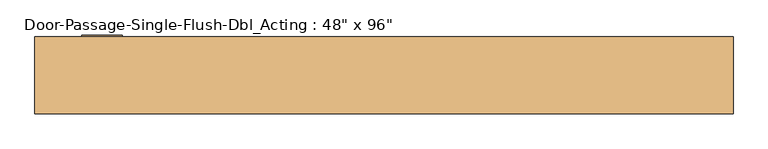
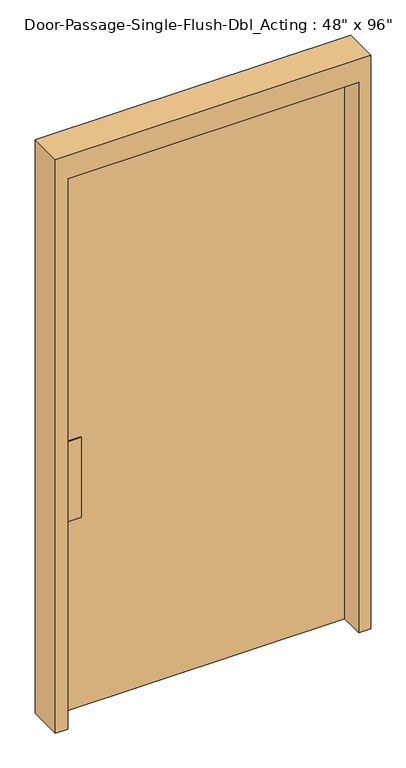
"""IFC4 building model written with IfcOpenShell, lengths in millimetres: door geometry."""

from ifc_helpers import new_model, si_unit, frame, origin, origin_with_axes, place, context, project, spatial, polyline, outline, extrude, source, transform, mapped, element, save


def door_bb6275b8(model_context):
    return source(origin(), model_context, "Body", "SweptSolid", [
        extrude(outline(polyline([(-571.5, 85.725), (-571.5, 88.9), (-495.3, 88.9), (-495.3, 85.725), (-571.5, 85.725)])), frame((0.0, 0.0, 838.2), z_axis=(0.0, 0.0, 1.0), x_axis=(1.0, 0.0, 0.0)), (0.0, 0.0, 1.0), 355.6),
        extrude(outline(polyline([(-571.5, 136.525), (-495.3, 136.525), (-495.3, 133.35), (-571.5, 133.35), (-571.5, 136.525)])), frame((0.0, 0.0, 838.2), z_axis=(0.0, 0.0, 1.0), x_axis=(1.0, 0.0, 0.0)), (0.0, 0.0, 1.0), 355.6),
        extrude(outline(polyline([(0.0, 609.6), (0.0, 660.4), (2540.0, 660.4), (2540.0, -660.4), (0.0, -660.4), (0.0, -609.6), (2438.4, -609.6), (2438.4, 609.6), (0.0, 609.6)])), frame((0.0, -12.7, 0.0), z_axis=(0.0, 1.0, 0.0), x_axis=(0.0, 0.0, 1.0)), (0.0, 0.0, 1.0), 146.05),
        extrude(outline(polyline([(609.6, 88.9), (-609.6, 88.9), (-609.6, 133.35), (609.6, 133.35), (609.6, 88.9)])), origin_with_axes(), (0.0, 0.0, 1.0), 2438.4),
    ])


if __name__ == "__main__":
    model = new_model("IFC4")
    model_context = context("Model", 3, world=origin())
    ifc_project = project(units=[si_unit("LENGTHUNIT", "METRE", prefix="MILLI")], contexts=[model_context])
    site = spatial("IfcSite", under=ifc_project)
    building = spatial("IfcBuilding", under=site)
    placement = place(None, origin())
    door_shape = door_bb6275b8(model_context)
    element("IfcDoor", 1, ObjectType="Door-Passage-Single-Flush-Dbl_Acting : 48\" x 96\"", at=placement, inside=building, context=model_context, shape_type="MappedRepresentation", body=[
        mapped(door_shape, transform((0.0, 0.0, 0.0), x_axis=(1.0, 0.0, 0.0), y_axis=(0.0, 1.0, 0.0), z_axis=(0.0, 0.0, 1.0))),
    ])
    save(model, "model.ifc")

# Revit data of these elements
# Type "Door-Passage-Single-Flush-Dbl_Acting : 48\" x 96\""
#   Type Mark = "8"
#   Assembly Code = "B2030200"
#   Analytic Construction = "Wooden"
#   Thickness = 0' - 1 3/4"
#   Thermal Resistance (R) = 2.5876 (h·ft²·°F)/BTU
#   Swing Angle [instance default] = 45.00°
#   Strike Height = 3' - 4"
#   Rough Width [instance default] = 4' - 4"
#   Rough Height [instance default] = 8' - 4"
#   MF Opening Height [instance default] = 0' - 4"
#   MF Opening Width [instance default] = 0' - 4"
#   Inset Calculate [instance default] = 0' - 4"
#   Masonry Inset [instance default] = 0' - 1"
#   Height = 8' - 0"
#   Width = 4' - 0"
#   Heat Transfer Coefficient (U) = 0.3865 BTU/(h·ft²·°F)
#   Masonry Frame Depth = 0' - 5 3/4"
#   Masonry Frame [instance default] = yes
#   Function = 1
#   Dry Wall Frame [instance default] = no
#   Panel Material = Wood - Birch
#   Frame Material = Metal - Paint Finish - Grey
#   Door Handle Material = Aluminum
#   Visual Light Transmittance = 0
#   Solar Heat Gain Coefficient = 0
#   Wall Closure = (empty or 0)
# Element 1 (IfcDoor, "Door-Passage-Single-Flush-Dbl_Acting : 48\" x 96\"")
#   Materials on its faces: "Aluminum", "Metal - Paint Finish - Grey", "Wood - Birch"
# Materials
#   "Wood - Birch": class "Wood", colour RGB 166 116 52, transparency 0, Cost = 0
#   "Metal - Paint Finish - Grey": class "Paint", colour RGB 104 104 104, transparency 0, Cost = 0
#   "Aluminum": class "Metal", colour RGB 247 247 247, transparency 0, Description = "Aluminum 6061", Cost = 0
